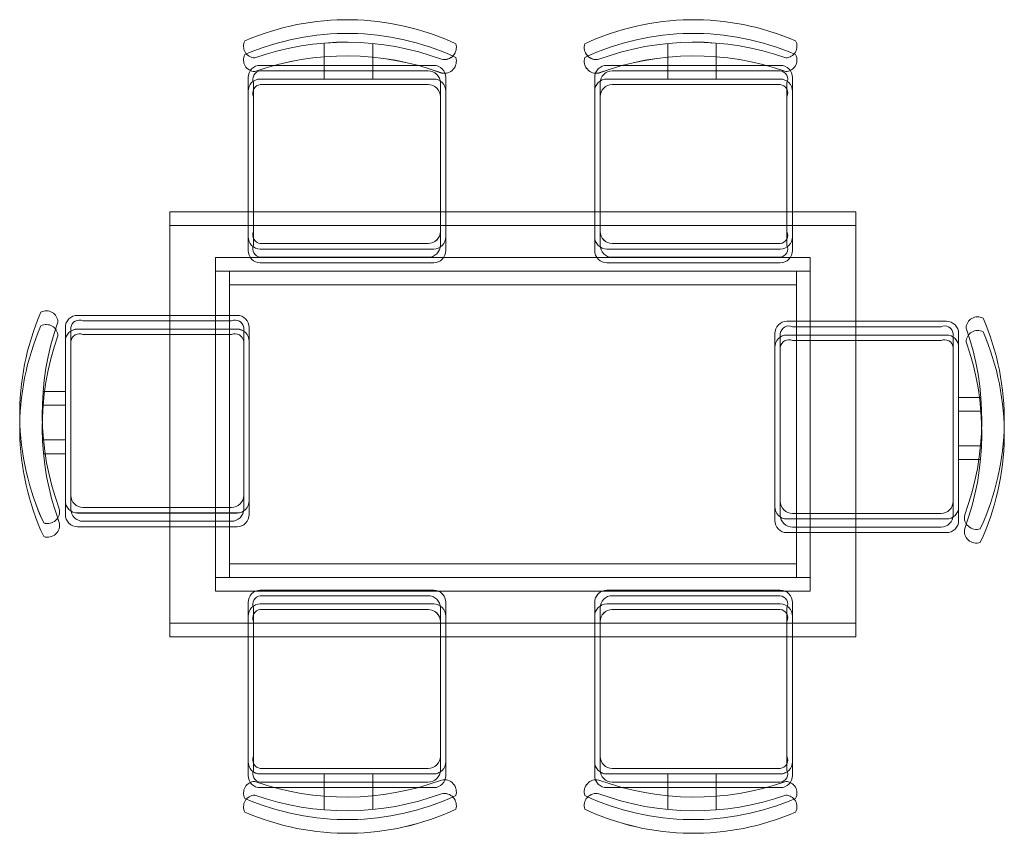
# Model space of a CAD drawing. Units: inches. Extents: x 963 to 2075, y 289 to 2657.
# Tile 62 of 98: x 1213 to 1264, y 2240 to 2283. Entities that reach past the tile are written whole.
import ezdxf

# ---------------------------------------------------------------- set-up
doc = ezdxf.new("R2010")
doc.units = ezdxf.units.IN
doc.layers.add('A-FURN', color=8, linetype='Continuous', lineweight=18)

msp = doc.modelspace()

# ---------------------------------------------------------------- linework, layer by layer
at = {"layer": 'A-FURN'}
for points in [[(1225.116, 2280.568, -0.175809), (1234.87, 2280.494, 0.578392), (1235.609, 2281.306, 0.214524), (1224.599, 2281.454, 0.552014), (1225.116, 2280.568, -0.065079)], [(1225.116, 2280.567, -0.175809), (1234.87, 2280.493, 0.578392), (1235.609, 2281.306, 0.214524), (1224.599, 2281.454, 0.552014), (1225.116, 2280.567, -0.065079)], [(1243.082, 2280.494, -0.578392), (1242.343, 2281.306, -0.214524), (1253.353, 2281.454, -0.552014), (1252.836, 2280.568, 0.175809), (1243.082, 2280.494)], [(1243.082, 2280.493, -0.578392), (1242.343, 2281.306, -0.214524), (1253.353, 2281.454, -0.552014), (1252.836, 2280.567, 0.175809), (1243.082, 2280.493)], [(1225.116, 2279.851, -0.175809), (1234.87, 2279.778, 0.578392), (1235.609, 2280.59, 0.214524), (1224.599, 2280.738, 0.552014), (1225.116, 2279.851, -0.065079)], [(1225.116, 2279.851, -0.175809), (1234.87, 2279.777, 0.578392), (1235.609, 2280.59, 0.214524), (1224.599, 2280.737, 0.552014), (1225.116, 2279.851, -0.065079)], [(1243.082, 2279.778, -0.578392), (1242.343, 2280.59, -0.214524), (1253.353, 2280.738, -0.552014), (1252.836, 2279.851, 0.175809), (1243.082, 2279.778)], [(1243.082, 2279.777, -0.578392), (1242.343, 2280.59, -0.214524), (1253.353, 2280.737, -0.552014), (1252.836, 2279.851, 0.175809), (1243.082, 2279.777)], [(1231.276, 2280.176), (1231.276, 2281.321, -0.064759)], [(1231.276, 2280.176), (1231.276, 2281.321, -0.064759)], [(1246.676, 2280.176), (1246.676, 2281.321, 0.064759)], [(1246.676, 2280.176), (1246.676, 2281.321, 0.064759)], [(1231.276, 2279.46), (1231.276, 2280.605, -0.064759)], [(1231.276, 2279.46), (1231.276, 2280.605, -0.064759)], [(1246.676, 2279.46), (1246.676, 2280.605, 0.064759)], [(1246.676, 2279.46), (1246.676, 2280.605, 0.064759)], [(1234.456, 2280.176), (1225.401, 2280.176, 0.414214), (1224.768, 2279.543), (1224.768, 2271.217, 0.414214), (1225.401, 2270.583), (1234.456, 2270.583, 0.414214), (1235.09, 2271.217), (1235.09, 2279.543, 0.414214), (1234.456, 2280.176)], [(1234.456, 2280.176), (1225.401, 2280.176, 0.414214), (1224.768, 2279.542), (1224.768, 2271.216, 0.414214), (1225.401, 2270.583), (1234.456, 2270.583, 0.414214), (1235.09, 2271.216), (1235.09, 2279.542, 0.414214), (1234.456, 2280.176)], [(1252.551, 2280.176, -0.414214), (1253.184, 2279.543), (1253.184, 2271.217, -0.414214), (1252.551, 2270.583), (1243.496, 2270.583, -0.414214), (1242.862, 2271.217), (1242.862, 2279.543, -0.414214), (1243.496, 2280.176), (1252.551, 2280.176)], [(1252.551, 2280.176, -0.414214), (1253.184, 2279.542), (1253.184, 2271.216, -0.414214), (1252.551, 2270.583), (1243.496, 2270.583, -0.414214), (1242.862, 2271.216), (1242.862, 2279.542, -0.414214), (1243.496, 2280.176), (1252.551, 2280.176)], [(1234.456, 2279.46), (1225.401, 2279.46, 0.414214), (1224.768, 2278.826), (1224.768, 2270.5, 0.414214), (1225.401, 2269.867), (1234.456, 2269.867, 0.414214), (1235.09, 2270.5), (1235.09, 2278.826, 0.414214), (1234.456, 2279.46)], [(1234.456, 2279.46), (1225.401, 2279.46, 0.414214), (1224.768, 2278.826), (1224.768, 2270.5, 0.414214), (1225.401, 2269.867), (1234.456, 2269.867, 0.414214), (1235.09, 2270.5), (1235.09, 2278.826, 0.414214), (1234.456, 2279.46)], [(1252.551, 2279.46, -0.414214), (1253.184, 2278.826), (1253.184, 2270.5, -0.414214), (1252.551, 2269.867), (1243.496, 2269.867, -0.414214), (1242.862, 2270.5), (1242.862, 2278.826, -0.414214), (1243.496, 2279.46), (1252.551, 2279.46)], [(1252.551, 2279.46, -0.414214), (1253.184, 2278.826), (1253.184, 2270.5, -0.414214), (1252.551, 2269.867), (1243.496, 2269.867, -0.414214), (1242.862, 2270.5), (1242.862, 2278.826, -0.414214), (1243.496, 2279.46), (1252.551, 2279.46)], [(1214.912, 2257.013, -0.578392), (1214.099, 2256.275, -0.214524), (1213.952, 2267.285, -0.552014), (1214.838, 2266.767, 0.175809), (1214.912, 2257.013)], [(1214.912, 2257.013, -0.578392), (1214.099, 2256.274, -0.214524), (1213.952, 2267.284, -0.552014), (1214.838, 2266.767, 0.175809), (1214.912, 2257.013)], [(1215.229, 2266.482, -0.414214), (1215.863, 2267.116), (1224.189, 2267.116, -0.414214), (1224.823, 2266.482), (1224.823, 2257.427, -0.414214), (1224.189, 2256.794), (1215.863, 2256.794, -0.414214), (1215.229, 2257.427), (1215.229, 2266.482)], [(1215.23, 2266.482, -0.414214), (1215.863, 2267.116), (1224.189, 2267.116, -0.414214), (1224.823, 2266.482), (1224.823, 2257.427, -0.414214), (1224.189, 2256.793), (1215.863, 2256.793, -0.414214), (1215.23, 2257.427), (1215.23, 2266.482)], [(1262.251, 2266.457, -0.175809), (1262.177, 2256.703, 0.578392), (1262.99, 2255.964, 0.214524), (1263.137, 2266.975, 0.552014), (1262.251, 2266.457, -0.065079)], [(1262.251, 2266.457, -0.175809), (1262.177, 2256.703, 0.578392), (1262.99, 2255.964, 0.214524), (1263.137, 2266.974, 0.552014), (1262.251, 2266.457, -0.065079)], [(1214.912, 2256.297, -0.578392), (1214.099, 2255.558, -0.214524), (1213.952, 2266.568, -0.552014), (1214.838, 2266.051, 0.175809), (1214.912, 2256.297)], [(1214.912, 2256.297, -0.578392), (1214.099, 2255.558, -0.214524), (1213.952, 2266.568, -0.552014), (1214.838, 2266.051, 0.175809), (1214.912, 2256.297)], [(1215.229, 2265.766, -0.414214), (1215.863, 2266.4), (1224.189, 2266.4, -0.414214), (1224.823, 2265.766), (1224.823, 2256.711, -0.414214), (1224.189, 2256.078), (1215.863, 2256.078, -0.414214), (1215.229, 2256.711), (1215.229, 2265.766)], [(1215.23, 2265.766, -0.414214), (1215.863, 2266.399), (1224.189, 2266.399, -0.414214), (1224.823, 2265.766), (1224.823, 2256.711, -0.414214), (1224.189, 2256.077), (1215.863, 2256.077, -0.414214), (1215.23, 2256.711), (1215.23, 2265.766)], [(1261.86, 2266.172, 0.414214), (1261.226, 2266.806), (1252.9, 2266.806, 0.414214), (1252.266, 2266.172), (1252.266, 2257.117, 0.414214), (1252.9, 2256.484), (1261.226, 2256.484, 0.414214), (1261.86, 2257.117), (1261.86, 2266.172)], [(1261.86, 2266.172, 0.414214), (1261.226, 2266.806), (1252.9, 2266.806, 0.414214), (1252.266, 2266.172), (1252.266, 2257.117, 0.414214), (1252.9, 2256.483), (1261.226, 2256.483, 0.414214), (1261.86, 2257.117), (1261.86, 2266.172)], [(1261.86, 2265.456, 0.414214), (1261.226, 2266.09), (1252.9, 2266.09, 0.414214), (1252.266, 2265.456), (1252.266, 2256.401, 0.414214), (1252.9, 2255.767), (1261.226, 2255.767, 0.414214), (1261.86, 2256.401), (1261.86, 2265.456)], [(1261.86, 2265.456, 0.414214), (1261.226, 2266.089), (1252.9, 2266.089, 0.414214), (1252.266, 2265.456), (1252.266, 2256.401, 0.414214), (1252.9, 2255.767), (1261.226, 2255.767, 0.414214), (1261.86, 2256.401), (1261.86, 2265.456)], [(1262.251, 2265.741, -0.175809), (1262.177, 2255.987, 0.578392), (1262.99, 2255.248, 0.214524), (1263.137, 2266.258, 0.552014), (1262.251, 2265.741, -0.065079)], [(1262.251, 2265.741, -0.175809), (1262.177, 2255.987, 0.578392), (1262.99, 2255.248, 0.214524), (1263.137, 2266.258, 0.552014), (1262.251, 2265.741, -0.065079)], [(1215.229, 2260.608), (1214.084, 2260.608, 0.064759)], [(1215.23, 2260.608), (1214.084, 2260.608, 0.064759)], [(1261.86, 2260.298), (1263.005, 2260.298, -0.064759)], [(1261.86, 2260.297), (1263.005, 2260.297, -0.064759)], [(1215.229, 2259.892), (1214.084, 2259.892, 0.064759)], [(1215.23, 2259.891), (1214.084, 2259.891, 0.064759)], [(1261.86, 2259.582), (1263.005, 2259.582, -0.064759)], [(1261.86, 2259.581), (1263.005, 2259.581, -0.064759)], [(1234.456, 2243.165), (1225.401, 2243.165, -0.414214), (1224.768, 2243.798), (1224.768, 2252.124, -0.414214), (1225.401, 2252.758), (1234.456, 2252.758, -0.414214), (1235.09, 2252.124), (1235.09, 2243.798, -0.414214), (1234.456, 2243.165)], [(1234.456, 2243.164), (1225.401, 2243.164, -0.414214), (1224.768, 2243.798), (1224.768, 2252.124, -0.414214), (1225.401, 2252.757), (1234.456, 2252.757, -0.414214), (1235.09, 2252.124), (1235.09, 2243.798, -0.414214), (1234.456, 2243.164)], [(1252.551, 2243.165, 0.414214), (1253.184, 2243.798), (1253.184, 2252.124, 0.414214), (1252.551, 2252.758), (1243.496, 2252.758, 0.414214), (1242.862, 2252.124), (1242.862, 2243.798, 0.414214), (1243.496, 2243.165), (1252.551, 2243.165)], [(1252.551, 2243.164, 0.414214), (1253.184, 2243.798), (1253.184, 2252.124, 0.414214), (1252.551, 2252.757), (1243.496, 2252.757, 0.414214), (1242.862, 2252.124), (1242.862, 2243.798, 0.414214), (1243.496, 2243.164), (1252.551, 2243.164)], [(1234.456, 2242.449), (1225.401, 2242.449, -0.414214), (1224.768, 2243.082), (1224.768, 2251.408, -0.414214), (1225.401, 2252.042), (1234.456, 2252.042, -0.414214), (1235.09, 2251.408), (1235.09, 2243.082, -0.414214), (1234.456, 2242.449)], [(1234.456, 2242.448), (1225.401, 2242.448, -0.414214), (1224.768, 2243.082), (1224.768, 2251.408, -0.414214), (1225.401, 2252.041), (1234.456, 2252.041, -0.414214), (1235.09, 2251.408), (1235.09, 2243.082, -0.414214), (1234.456, 2242.448)], [(1252.551, 2242.449, 0.414214), (1253.184, 2243.082), (1253.184, 2251.408, 0.414214), (1252.551, 2252.042), (1243.496, 2252.042, 0.414214), (1242.862, 2251.408), (1242.862, 2243.082, 0.414214), (1243.496, 2242.449), (1252.551, 2242.449)], [(1252.551, 2242.448, 0.414214), (1253.184, 2243.082), (1253.184, 2251.408, 0.414214), (1252.551, 2252.041), (1243.496, 2252.041, 0.414214), (1242.862, 2251.408), (1242.862, 2243.082, 0.414214), (1243.496, 2242.448), (1252.551, 2242.448)], [(1234.87, 2242.847, -0.578392), (1235.609, 2242.035, -0.214524), (1224.599, 2241.887, -0.552014), (1225.116, 2242.773, 0.175809), (1234.87, 2242.847)], [(1234.87, 2242.847, -0.578392), (1235.609, 2242.034, -0.214524), (1224.599, 2241.886, -0.552014), (1225.116, 2242.773, 0.175809), (1234.87, 2242.847)], [(1231.276, 2243.165), (1231.276, 2242.02, 0.064759)], [(1231.276, 2243.164), (1231.276, 2242.019, 0.064759)], [(1252.836, 2242.773, -0.175809), (1243.082, 2242.847, 0.578392), (1242.343, 2242.035, 0.214524), (1253.353, 2241.887, 0.552014), (1252.836, 2242.773, -0.065079)], [(1252.836, 2242.773, -0.175809), (1243.082, 2242.847, 0.578392), (1242.343, 2242.034, 0.214524), (1253.353, 2241.886, 0.552014), (1252.836, 2242.773, -0.065079)], [(1246.676, 2243.165), (1246.676, 2242.02, -0.064759)], [(1246.676, 2243.164), (1246.676, 2242.019, -0.064759)], [(1231.276, 2242.449), (1231.276, 2241.303, 0.064759)], [(1231.276, 2242.448), (1231.276, 2241.303, 0.064759)], [(1246.676, 2242.449), (1246.676, 2241.303, -0.064759)], [(1246.676, 2242.448), (1246.676, 2241.303, -0.064759)], [(1234.87, 2242.131, -0.578392), (1235.609, 2241.318, -0.214524), (1224.599, 2241.171, -0.552014), (1225.116, 2242.057, 0.175809), (1234.87, 2242.131)], [(1234.87, 2242.131, -0.578392), (1235.609, 2241.318, -0.214524), (1224.599, 2241.17, -0.552014), (1225.116, 2242.057, 0.175809), (1234.87, 2242.131)], [(1252.836, 2242.057, -0.175809), (1243.082, 2242.131, 0.578392), (1242.343, 2241.318, 0.214524), (1253.353, 2241.171, 0.552014), (1252.836, 2242.057, -0.065079)], [(1252.836, 2242.057, -0.175809), (1243.082, 2242.131, 0.578392), (1242.343, 2241.318, 0.214524), (1253.353, 2241.17, 0.552014), (1252.836, 2242.057, -0.065079)]]:
    msp.add_lwpolyline(points, format="xyb", dxfattribs=at)
for points in [[(1228.741, 2281.342), (1228.741, 2280.176)], [(1228.741, 2281.342), (1228.741, 2280.176)], [(1249.211, 2281.342), (1249.211, 2280.176)], [(1249.211, 2281.342), (1249.211, 2280.176)], [(1228.741, 2280.626), (1228.741, 2279.46)], [(1228.741, 2280.626), (1228.741, 2279.46)], [(1249.211, 2280.626), (1249.211, 2279.46)], [(1249.211, 2280.626), (1249.211, 2279.46)], [(1214.063, 2263.143), (1215.229, 2263.143)], [(1214.063, 2263.142), (1215.23, 2263.142)], [(1263.026, 2262.832), (1261.86, 2262.832)], [(1263.026, 2262.832), (1261.86, 2262.832)], [(1214.063, 2262.426), (1215.229, 2262.426)], [(1214.063, 2262.426), (1215.23, 2262.426)], [(1263.026, 2262.116), (1261.86, 2262.116)], [(1263.026, 2262.116), (1261.86, 2262.116)], [(1228.741, 2241.999), (1228.741, 2243.165)], [(1228.741, 2241.998), (1228.741, 2243.164)], [(1249.211, 2241.999), (1249.211, 2243.165)], [(1249.211, 2241.998), (1249.211, 2243.164)], [(1228.741, 2241.282), (1228.741, 2242.449)], [(1228.741, 2241.282), (1228.741, 2242.448)], [(1249.211, 2241.282), (1249.211, 2242.449)], [(1249.211, 2241.282), (1249.211, 2242.448)]]:
    msp.add_lwpolyline(points, dxfattribs=at)
for points in [[(1225.405, 2279.891), (1234.171, 2279.891, -0.414214), (1234.805, 2279.257), (1234.805, 2271.502, -0.414214), (1234.171, 2270.869), (1225.405, 2270.869, -0.512069), (1225.053, 2271.502), (1225.053, 2279.257, -0.512069)], [(1225.405, 2279.89), (1234.171, 2279.89, -0.414214), (1234.805, 2279.257), (1234.805, 2271.502, -0.414214), (1234.171, 2270.868), (1225.405, 2270.868, -0.512069), (1225.053, 2271.502), (1225.053, 2279.257, -0.512069)], [(1252.547, 2279.891), (1243.781, 2279.891, 0.414214), (1243.147, 2279.257), (1243.147, 2271.502, 0.414214), (1243.781, 2270.869), (1252.547, 2270.869, 0.512069), (1252.899, 2271.502), (1252.899, 2279.257, 0.512069)], [(1252.547, 2279.89), (1243.781, 2279.89, 0.414214), (1243.148, 2279.257), (1243.148, 2271.502, 0.414214), (1243.781, 2270.868), (1252.547, 2270.868, 0.512069), (1252.899, 2271.502), (1252.899, 2279.257, 0.512069)], [(1225.405, 2279.175), (1234.171, 2279.175, -0.414214), (1234.805, 2278.541), (1234.805, 2270.786, -0.414214), (1234.171, 2270.152), (1225.405, 2270.152, -0.512069), (1225.053, 2270.786), (1225.053, 2278.541, -0.512069)], [(1225.405, 2279.174), (1234.171, 2279.174, -0.414214), (1234.805, 2278.541), (1234.805, 2270.785, -0.414214), (1234.171, 2270.152), (1225.405, 2270.152, -0.512069), (1225.053, 2270.785), (1225.053, 2278.541, -0.512069)], [(1252.547, 2279.175), (1243.781, 2279.175, 0.414214), (1243.147, 2278.541), (1243.147, 2270.786, 0.414214), (1243.781, 2270.152), (1252.547, 2270.152, 0.512069), (1252.899, 2270.786), (1252.899, 2278.541, 0.512069)], [(1252.547, 2279.174), (1243.781, 2279.174, 0.414214), (1243.148, 2278.541), (1243.148, 2270.785, 0.414214), (1243.781, 2270.152), (1252.547, 2270.152, 0.512069), (1252.899, 2270.785), (1252.899, 2278.541, 0.512069)], [(1215.515, 2266.479), (1215.515, 2257.713, 0.414214), (1216.148, 2257.079), (1223.904, 2257.079, 0.414214), (1224.537, 2257.713), (1224.537, 2266.479, 0.512069), (1223.904, 2266.831), (1216.148, 2266.831, 0.512069)], [(1215.515, 2266.478), (1215.515, 2257.712, 0.414214), (1216.148, 2257.079), (1223.904, 2257.079, 0.414214), (1224.537, 2257.712), (1224.537, 2266.478, 0.512069), (1223.904, 2266.83), (1216.148, 2266.83, 0.512069)], [(1261.574, 2266.169), (1261.574, 2257.403, -0.414214), (1260.941, 2256.769), (1253.185, 2256.769, -0.414214), (1252.552, 2257.403), (1252.552, 2266.169, -0.512069), (1253.185, 2266.52), (1260.941, 2266.52, -0.512069)], [(1261.574, 2266.168), (1261.574, 2257.402, -0.414214), (1260.941, 2256.769), (1253.185, 2256.769, -0.414214), (1252.552, 2257.402), (1252.552, 2266.168, -0.512069), (1253.185, 2266.52), (1260.941, 2266.52, -0.512069)], [(1215.515, 2265.762), (1215.515, 2256.996, 0.414214), (1216.148, 2256.363), (1223.904, 2256.363, 0.414214), (1224.537, 2256.996), (1224.537, 2265.762, 0.512069), (1223.904, 2266.114), (1216.148, 2266.114, 0.512069)], [(1215.515, 2265.762), (1215.515, 2256.996, 0.414214), (1216.148, 2256.363), (1223.904, 2256.363, 0.414214), (1224.537, 2256.996), (1224.537, 2265.762, 0.512069), (1223.904, 2266.114), (1216.148, 2266.114, 0.512069)], [(1261.574, 2265.452), (1261.574, 2256.686, -0.414214), (1260.941, 2256.053), (1253.185, 2256.053, -0.414214), (1252.552, 2256.686), (1252.552, 2265.452, -0.512069), (1253.185, 2265.804), (1260.941, 2265.804, -0.512069)], [(1261.574, 2265.452), (1261.574, 2256.686, -0.414214), (1260.941, 2256.052), (1253.185, 2256.052, -0.414214), (1252.552, 2256.686), (1252.552, 2265.452, -0.512069), (1253.185, 2265.804), (1260.941, 2265.804, -0.512069)], [(1225.405, 2243.45), (1234.171, 2243.45, 0.414214), (1234.805, 2244.084), (1234.805, 2251.839, 0.414214), (1234.171, 2252.472), (1225.405, 2252.472, 0.512069), (1225.053, 2251.839), (1225.053, 2244.084, 0.512069)], [(1225.405, 2243.45), (1234.171, 2243.45, 0.414214), (1234.805, 2244.083), (1234.805, 2251.839, 0.414214), (1234.171, 2252.472), (1225.405, 2252.472, 0.512069), (1225.053, 2251.839), (1225.053, 2244.083, 0.512069)], [(1252.547, 2243.45), (1243.781, 2243.45, -0.414214), (1243.147, 2244.084), (1243.147, 2251.839, -0.414214), (1243.781, 2252.472), (1252.547, 2252.472, -0.512069), (1252.899, 2251.839), (1252.899, 2244.084, -0.512069)], [(1252.547, 2243.45), (1243.781, 2243.45, -0.414214), (1243.148, 2244.083), (1243.148, 2251.839, -0.414214), (1243.781, 2252.472), (1252.547, 2252.472, -0.512069), (1252.899, 2251.839), (1252.899, 2244.083, -0.512069)], [(1225.405, 2242.734), (1234.171, 2242.734, 0.414214), (1234.805, 2243.367), (1234.805, 2251.123, 0.414214), (1234.171, 2251.756), (1225.405, 2251.756, 0.512069), (1225.053, 2251.123), (1225.053, 2243.367, 0.512069)], [(1225.405, 2242.734), (1234.171, 2242.734, 0.414214), (1234.805, 2243.367), (1234.805, 2251.122, 0.414214), (1234.171, 2251.756), (1225.405, 2251.756, 0.512069), (1225.053, 2251.122), (1225.053, 2243.367, 0.512069)], [(1252.547, 2242.734), (1243.781, 2242.734, -0.414214), (1243.147, 2243.367), (1243.147, 2251.123, -0.414214), (1243.781, 2251.756), (1252.547, 2251.756, -0.512069), (1252.899, 2251.123), (1252.899, 2243.367, -0.512069)], [(1252.547, 2242.734), (1243.781, 2242.734, -0.414214), (1243.148, 2243.367), (1243.148, 2251.122, -0.414214), (1243.781, 2251.756), (1252.547, 2251.756, -0.512069), (1252.899, 2251.122), (1252.899, 2243.367, -0.512069)]]:
    msp.add_lwpolyline(points, format="xyb", close=True, dxfattribs=at)
for points in [[(1220.687, 2272.529), (1256.498, 2272.529), (1256.498, 2251.042), (1220.687, 2251.042)], [(1220.687, 2272.528), (1256.498, 2272.528), (1256.498, 2251.042), (1220.687, 2251.042)], [(1220.687, 2271.813), (1256.498, 2271.813), (1256.498, 2250.326), (1220.687, 2250.326)], [(1220.687, 2271.812), (1256.498, 2271.812), (1256.498, 2250.326), (1220.687, 2250.326)], [(1223.074, 2270.141), (1254.111, 2270.141), (1254.111, 2253.43), (1223.074, 2253.43)], [(1223.074, 2270.141), (1254.111, 2270.141), (1254.111, 2253.429), (1223.074, 2253.429)], [(1223.074, 2269.425), (1254.111, 2269.425), (1254.111, 2252.713), (1223.074, 2252.713)], [(1223.074, 2269.425), (1254.111, 2269.425), (1254.111, 2252.713), (1223.074, 2252.713)], [(1223.791, 2269.425), (1253.394, 2269.425), (1253.394, 2254.146), (1223.791, 2254.146)], [(1223.791, 2269.425), (1253.394, 2269.425), (1253.394, 2254.145), (1223.791, 2254.145)], [(1223.791, 2268.709), (1253.394, 2268.709), (1253.394, 2253.43), (1223.791, 2253.43)], [(1223.791, 2268.709), (1253.394, 2268.709), (1253.394, 2253.429), (1223.791, 2253.429)]]:
    msp.add_lwpolyline(points, close=True, dxfattribs=at)

doc.saveas('drawing.dxf')
